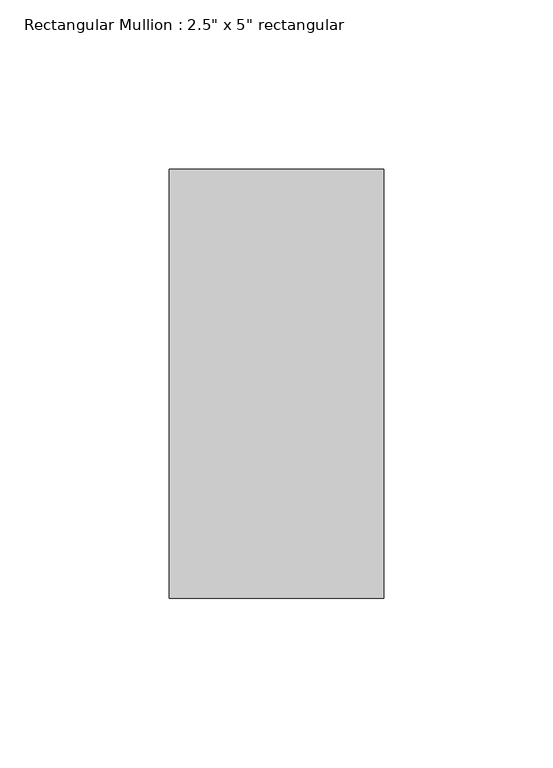
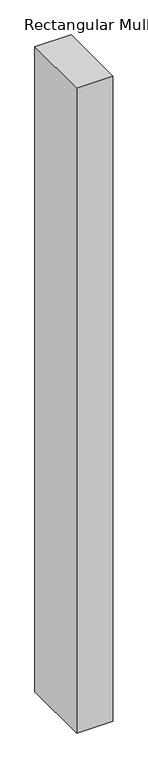
"""IFC4 building model written with IfcOpenShell, lengths in millimetres: member geometry."""

from ifc_helpers import new_model, si_unit, frame, origin, place, context, project, spatial, polyline, outline, extrude, source, transform, mapped, element, save


def member_fec1d5e2(model_context):
    return source(origin(), model_context, "Body", "SweptSolid", [
        extrude(outline(polyline([(31.75, 63.5), (31.75, -63.5), (-31.75, -63.5), (-31.75, 63.5), (31.75, 63.5)])), frame((0.0, 0.0, -1194.1019988), z_axis=(0.0, 0.0, 1.0), x_axis=(1.0, 0.0, 0.0)), (0.0, 0.0, 1.0), 1194.1019988),
    ])


if __name__ == "__main__":
    model = new_model("IFC4")
    model_context = context("Model", 3, world=origin())
    ifc_project = project(units=[si_unit("LENGTHUNIT", "METRE", prefix="MILLI")], contexts=[model_context])
    site = spatial("IfcSite", under=ifc_project)
    building = spatial("IfcBuilding", under=site)
    placement = place(None, origin())
    member_shape = member_fec1d5e2(model_context)
    element("IfcMember", 1, ObjectType="Rectangular Mullion : 2.5\" x 5\" rectangular", at=placement, inside=building, context=model_context, shape_type="MappedRepresentation", body=[
        mapped(member_shape, transform((0.0, 0.0, 0.0), x_axis=(1.0, 0.0, 0.0), y_axis=(0.0, 1.0, 0.0), z_axis=(0.0, 0.0, 1.0))),
    ])
    save(model, "model.ifc")

# Revit data of these elements
# Type "Rectangular Mullion : 2.5\" x 5\" rectangular"
#   built-in parameter 1007304 = 0.416667 (stored number, unit not read)
#   built-in parameter 1007301 = 0.104167 (stored number, unit not read)
#   built-in parameter 1007300 = 0.104167 (stored number, unit not read)
# Element 1 (IfcMember, "Rectangular Mullion : 2.5\" x 5\" rectangular")
#   Materials on its faces: "Aluminum"
# Materials
#   "Aluminum": class "Metal", colour RGB 247 247 247, transparency 0, Description = "Aluminum 6061", Cost = 0
